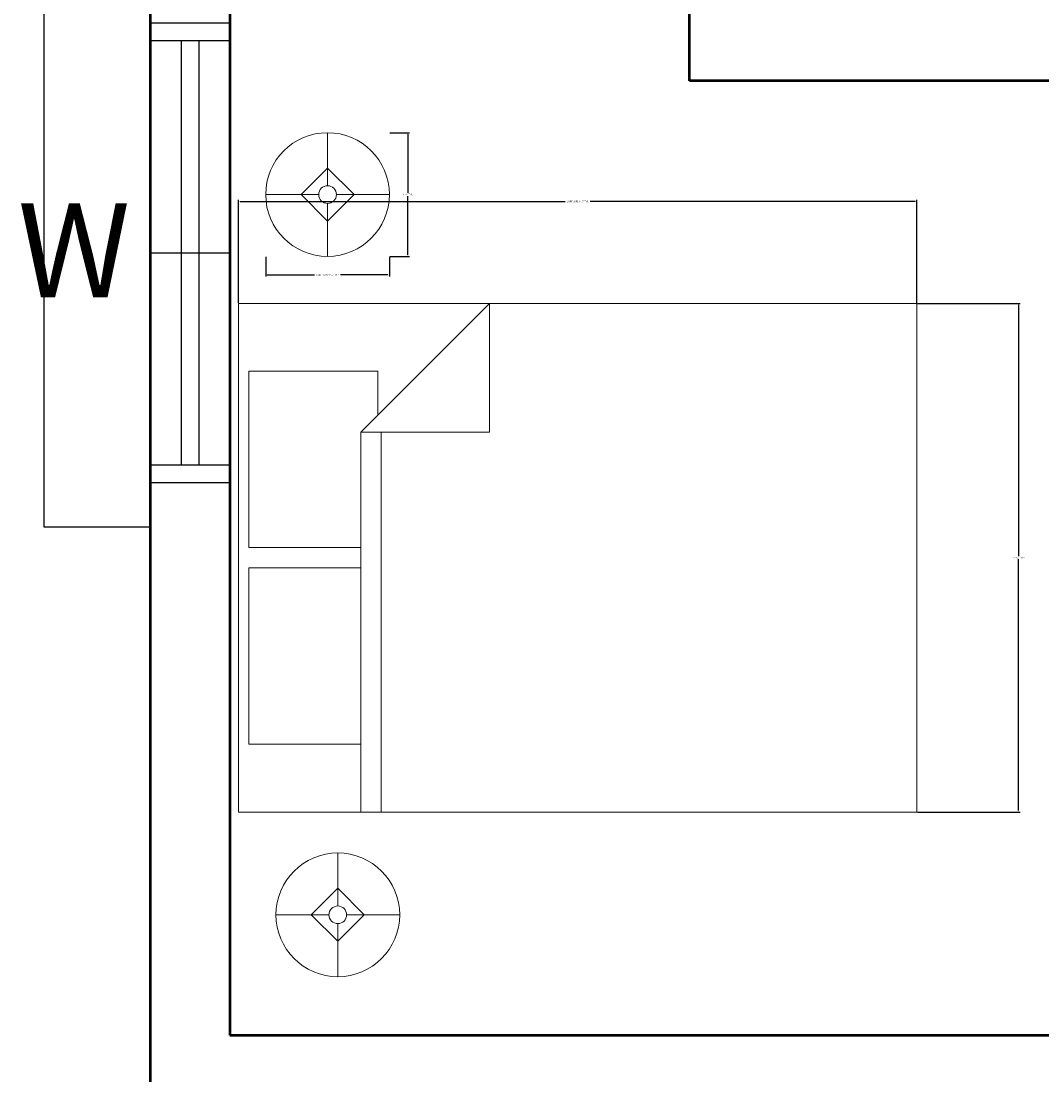
# Model space of a CAD drawing. Units: inches. Extents: x -105 to 1196, y -792 to 119.
# Tile 7 of 23: x -60 to 56, y -121 to -1. Entities that reach past the tile are written whole.
import ezdxf

# ---------------------------------------------------------------- set-up
doc = ezdxf.new("R2010")
doc.units = ezdxf.units.IN
doc.header["$MEASUREMENT"] = 0
for name, color, linetype, lineweight in [('A-ANNO-DIMS', 2, 'Continuous', 18), ('A-ANNO-TEXT', 7, 'Continuous', 25), ('A-FURN', 8, 'Continuous', 18), ('A-GLAZ', 4, 'Continuous', 25), ('A-WALL', 3, 'Continuous', 50)]:
    doc.layers.add(name, color=color, linetype=linetype, lineweight=lineweight)
doc.styles.get("Standard").update_dxf_attribs({"font": 'arial.ttf'})
doc.dimstyles.get("Standard").update_dxf_attribs({"dimtxt": 0.18, "dimasz": 0.18, "dimexe": 0.18, "dimexo": 0.0625, "dimgap": 0.09, "dimtad": 0, "dimtih": 1, "dimtoh": 1, "dimdec": 1, "dimzin": 0, "dimdsep": 46, "dimlunit": 4, "dimtxsty": 'Standard', "dimcen": 0.09, "dimadec": 0, "dimazin": 0, "dimtfac": 1, "dimtdec": 1, "dimtofl": 0, "dimtmove": 0, "dimatfit": 3, "dimfxl": 1, "dimtolj": 1, "dimtzin": 0, "dimarcsym": 0})

# ---------------------------------------------------------------- blocks, each defined once
blk = doc.blocks.new('Bed - Queen')
for p, q in [((0, -80.00003), (0, 0)), ((0, 0), (59.99999, 0)), ((59.99999, 0), (59.99999, -80.00003)), ((7.99999, -1.2), (28.79998, -1.2)), ((7.99999, -14.4), (7.99999, -1.2)), ((28.79998, -1.2), (28.79998, -14.4)), ((31.19999, -1.2), (51.99999, -1.2)), ((31.19999, -14.4), (31.19999, -1.2)), ((51.99999, -1.2), (51.99999, -16.4)), ((0, -14.4), (44.8, -14.4)), ((59.99999, -29.6), (44.8, -14.4)), ((44.8, -14.4), (44.8, -29.6)), ((44.8, -16.8), (0, -16.8)), ((51.99999, -16.4), (46.79936, -16.4)), ((44.8, -29.6), (59.99999, -29.6)), ((59.99999, -80.00003), (0, -80.00003))]:
    blk.add_line(p, q)
blk = doc.blocks.new('Lamp - Table')
for p, q in [((0, 7), (0, 1)), ((0, 3), (-3, 0)), ((3, 0), (0, 3)), ((-1, 0), (-7, 0)), ((-3, 0), (0, -3)), ((0, -3), (3, 0)), ((1, 0), (7, 0)), ((0, -1), (0, -7))]:
    blk.add_line(p, q)
for radius in [7, 1]:
    blk.add_circle((0, 0), radius)
blk = doc.blocks.new('WIN-1200')
at = {"ltscale": 2}
for p, q in [((12, 62), (0, 62)), ((0, 0), (0, 62)), ((12, 57), (12, 62)), ((12, 5), (12, 0)), ((12, 0), (0, 0))]:
    blk.add_line(p, q, dxfattribs=at)
for p, q in [((21, 57), (12, 57)), ((21, 5), (12, 5))]:
    blk.add_line(p, q)
blk = doc.blocks.new('*D59')
at = {"layer": 'A-ANNO-DIMS', "color": 0, "lineweight": -2, "transparency": 16777216}
for p, q in [((-35.26, -33.35), (-35.26, -21.72)), ((-35.08, -21.9), (1.7, -21.9)), ((41.31, -21.9), (4.53, -21.9)), ((41.49, -33.35), (41.49, -21.72))]:
    blk.add_line(p, q, dxfattribs=at)
at = {"layer": 'A-ANNO-DIMS', "color": 0, "transparency": 16777216}
for points in [[(-35.08, -21.87), (-35.08, -21.93), (-35.26, -21.9)], [(41.31, -21.87), (41.31, -21.93), (41.49, -21.9)]]:
    blk.add_solid(points, dxfattribs=at)
at = {"layer": 'Defpoints', "color": 0, "transparency": 16777216}
for p in [(-35.26, -21.9), (-35.26, -33.42), (41.49, -33.42)]:
    blk.add_point(p, dxfattribs=at)
at = {"layer": 'A-ANNO-DIMS', "color": 0, "transparency": 16777216, "insert": (3.11, -21.9), "char_height": 0.18, "attachment_point": 5}
blk.add_mtext('\\A1;QUEEN BED 6\'-5" TYP.', dxfattribs=at)
blk = doc.blocks.new('*D60')
at = {"layer": 'A-ANNO-DIMS', "color": 0, "lineweight": -2, "transparency": 16777216}
for p, q in [((41.55, -33.42), (53.18, -33.42)), ((53, -33.6), (53, -62.01)), ((53, -90.8), (53, -62.38)), ((41.55, -90.98), (53.18, -90.98))]:
    blk.add_line(p, q, dxfattribs=at)
at = {"layer": 'A-ANNO-DIMS', "color": 0, "transparency": 16777216}
for points in [[(52.97, -33.6), (53.03, -33.6), (53, -33.42)], [(52.97, -90.8), (53.03, -90.8), (53, -90.98)]]:
    blk.add_solid(points, dxfattribs=at)
at = {"layer": 'Defpoints', "color": 0, "transparency": 16777216}
for p in [(41.49, -33.42), (53, -33.42), (41.49, -90.98)]:
    blk.add_point(p, dxfattribs=at)
at = {"layer": 'A-ANNO-DIMS', "color": 0, "transparency": 16777216, "insert": (53, -62.2), "char_height": 0.18, "attachment_point": 5}
blk.add_mtext('\\A1;4\'-9 1/2" TYP.', dxfattribs=at)
blk = doc.blocks.new('*D71')
at = {"layer": 'A-ANNO-DIMS', "color": 0, "lineweight": -2, "transparency": 16777216}
for p, q in [((-32.2, -28.17), (-32.2, -30.39)), ((-18.2, -28.17), (-18.2, -30.39)), ((-32.02, -30.21), (-26.66, -30.21)), ((-18.38, -30.21), (-23.75, -30.21))]:
    blk.add_line(p, q, dxfattribs=at)
at = {"layer": 'A-ANNO-DIMS', "color": 0, "transparency": 16777216}
for points in [[(-32.02, -30.18), (-32.02, -30.24), (-32.2, -30.21)], [(-18.38, -30.18), (-18.38, -30.24), (-18.2, -30.21)]]:
    blk.add_solid(points, dxfattribs=at)
at = {"layer": 'Defpoints', "color": 0, "transparency": 16777216}
for p in [(-32.2, -28.11), (-18.2, -28.11), (-18.2, -30.21)]:
    blk.add_point(p, dxfattribs=at)
at = {"layer": 'A-ANNO-DIMS', "color": 0, "transparency": 16777216, "insert": (-25.2, -30.21), "char_height": 0.18, "attachment_point": 5}
blk.add_mtext('\\A1;TABLE LAMP 1\'-2" TYP.', dxfattribs=at)
blk = doc.blocks.new('*D72')
at = {"layer": 'A-ANNO-DIMS', "color": 0, "lineweight": -2, "transparency": 16777216}
for p, q in [((-18.14, -14.11), (-15.92, -14.11)), ((-16.1, -14.29), (-16.1, -20.93)), ((-16.1, -27.93), (-16.1, -21.29)), ((-18.14, -28.11), (-15.92, -28.11))]:
    blk.add_line(p, q, dxfattribs=at)
at = {"layer": 'A-ANNO-DIMS', "color": 0, "transparency": 16777216}
for points in [[(-16.13, -14.29), (-16.07, -14.29), (-16.1, -14.11)], [(-16.13, -27.93), (-16.07, -27.93), (-16.1, -28.11)]]:
    blk.add_solid(points, dxfattribs=at)
at = {"layer": 'Defpoints', "color": 0, "transparency": 16777216}
for p in [(-18.2, -14.11), (-16.1, -14.11), (-18.2, -28.11)]:
    blk.add_point(p, dxfattribs=at)
at = {"layer": 'A-ANNO-DIMS', "color": 0, "transparency": 16777216, "insert": (-16.1, -21.11), "char_height": 0.18, "attachment_point": 5}
blk.add_mtext('\\A1;1\'-2" TYP.', dxfattribs=at)

msp = doc.modelspace()

# ---------------------------------------------------------------- linework, layer by layer
at = {"layer": 'A-GLAZ'}
for p, q in [((-36.26, -3.73), (-45.26, -3.73)), ((-41.76, -3.73), (-41.76, -51.73)), ((-39.76, -3.73), (-39.76, -51.73)), ((-36.26, -27.73), (-45.26, -27.73)), ((-36.26, -51.73), (-45.26, -51.73))]:
    msp.add_line(p, q, dxfattribs=at)
at = {"layer": 'A-WALL'}
for p, q in [((-45.26, 69.77), (-45.26, -125.23)), ((-36.26, 60.77), (-36.26, -116.23)), ((15.74, -8.23), (15.74, 0.77)), ((48.74, -8.23), (15.74, -8.23)), ((120.74, -8.23), (48.74, -8.23)), ((-36.26, -116.23), (129.74, -116.23))]:
    msp.add_line(p, q, dxfattribs=at)

# ---------------------------------------------------------------- block references
at = {"layer": 'A-FURN'}
for p in [(-25.2, -21.11), (-24.04, -102.61)]:
    msp.add_blockref('Lamp - Table', p, dxfattribs=at)
at = {"layer": 'A-FURN', "xscale": 0.9593862173514477, "yscale": 0.9593862173514477, "zscale": 0.9593862173514477, "rotation": 90}
msp.add_blockref('Bed - Queen', (-35.26, -90.98), dxfattribs=at)
at = {"layer": 'A-GLAZ'}
msp.add_blockref('WIN-1200', (-57.26, -58.73), dxfattribs=at)

# ---------------------------------------------------------------- texts
at = {"layer": 'A-ANNO-TEXT'}
msp.add_text('W', height=10.64, dxfattribs=at).set_placement((-60.26, -32.75))

# ---------------------------------------------------------------- dimensions: what is measured, and where the dimension line sits
at = {"layer": 'A-ANNO-DIMS'}
for base, p1, p2, angle, text, picture, middle in [((-16.1, -14.11), (-18.2, -28.11), (-18.2, -14.11), 90, '<> TYP.', '*D72', (-16.1, -21.11)), ((-35.2634, -21.903), (41.4875, -33.4156), (-35.2634, -33.4156), 180, 'QUEEN BED <> TYP.', '*D59', (3.1121, -21.903)), ((53, -33.42), (41.49, -90.98), (41.49, -33.42), 90, '<> TYP.', '*D60', (53, -62.2))]:
    dim = msp.add_linear_dim(base=base, p1=p1, p2=p2, angle=angle, text=text, dimstyle='Standard', override={"dimdec": 1, "dimlfac": 1, "dimrnd": 0, "dimzin": 1, "dimdsep": 46, "dimlunit": 4, "dimfrac": 2}, dxfattribs=at)
    dim.commit()
    dim.dimension.update_dxf_attribs({"geometry": picture, "text_midpoint": middle})
dim = msp.add_linear_dim(base=(-18.2, -30.21), p1=(-32.2, -28.11), p2=(-18.2, -28.11), text='TABLE LAMP <> TYP.', dimstyle='Standard', override={"dimdec": 1, "dimlfac": 1, "dimrnd": 0, "dimzin": 1, "dimdsep": 46, "dimlunit": 4, "dimfrac": 2}, dxfattribs=at)
dim.commit()
dim.dimension.update_dxf_attribs({"geometry": '*D71', "text_midpoint": (-25.2, -30.21)})

doc.saveas('drawing.dxf')
